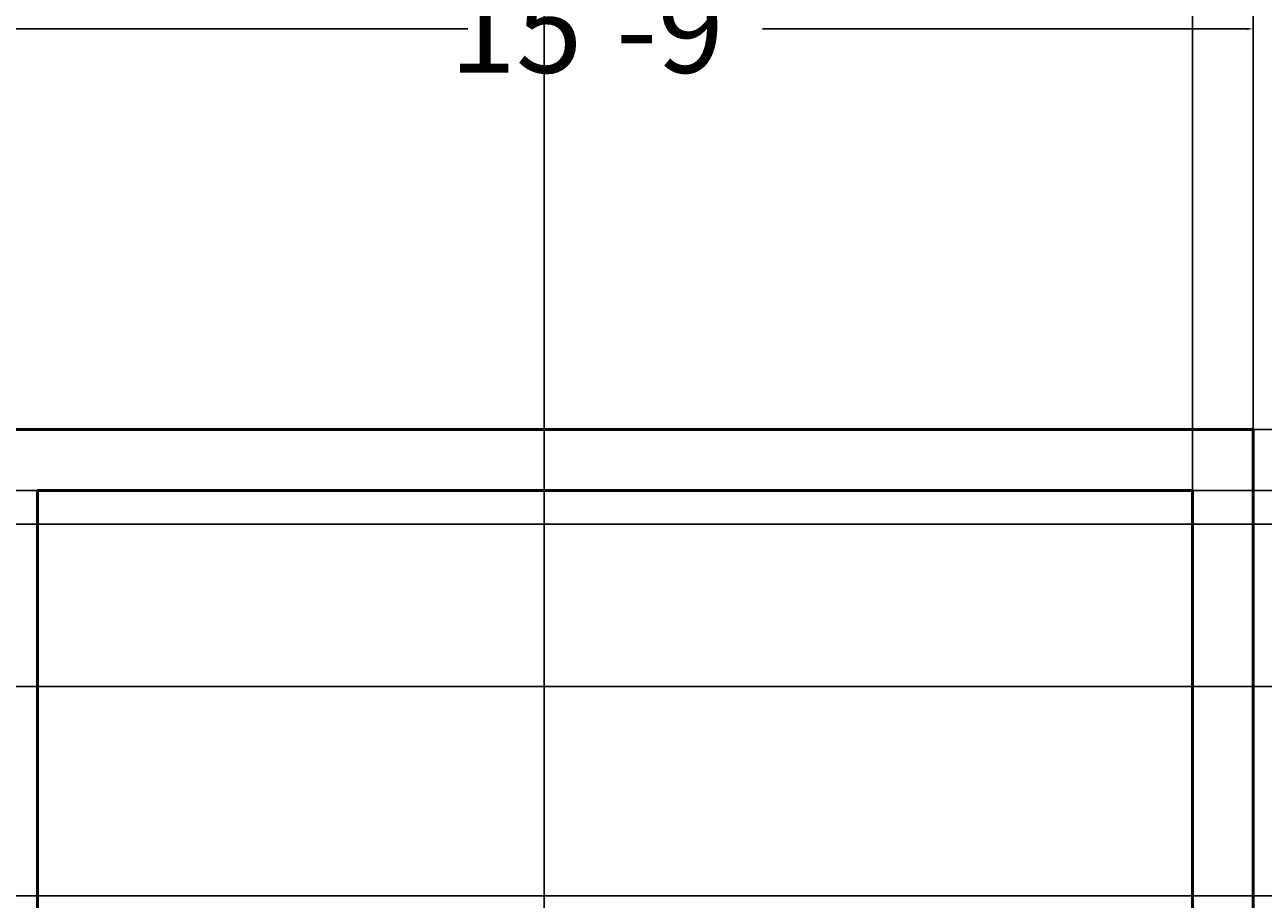
# Model space of a CAD drawing. Units: inches. Extents: x -364 to 705, y -52 to 1250.
# Tile 32 of 34: x 366 to 549, y 917 to 1046. Entities that reach past the tile are written whole.
import ezdxf

# ---------------------------------------------------------------- set-up
doc = ezdxf.new("R2010")
doc.units = ezdxf.units.IN
doc.header["$MEASUREMENT"] = 0
doc.layers.add('A-ANNO-DIMS', color=4, linetype='Continuous', lineweight=18)
doc.layers.add('A-WALL', color=41, linetype='Continuous', lineweight=50)
doc.styles.get("Standard").update_dxf_attribs({"font": 'arial.ttf'})
doc.dimstyles.get("Standard").update_dxf_attribs({"dimtxt": 1, "dimasz": 1, "dimexe": 0.18, "dimexo": 0.0625, "dimgap": 0.09, "dimtad": 0, "dimtih": 1, "dimtoh": 1, "dimdec": 0, "dimzin": 0, "dimdsep": 46, "dimlunit": 3, "dimtxsty": 'Standard', "dimcen": 0.09, "dimadec": 0, "dimazin": 0, "dimtfac": 1, "dimtdec": 0, "dimtofl": 0, "dimtmove": 0, "dimatfit": 3, "dimfxl": 1, "dimtolj": 1, "dimtzin": 0, "dimarcsym": 0})

# ---------------------------------------------------------------- blocks, each defined once
blk = doc.blocks.new('*D23')
at = {"layer": 'A-ANNO-DIMS', "color": 0, "lineweight": -2, "transparency": 16777216}
for p, q in [((28.58, 986.18), (28.58, 1127.53)), ((29.58, 1127.35), (265.4, 1127.35)), ((546.58, 1127.35), (310.76, 1127.35)), ((547.58, 986.18), (547.58, 1127.53))]:
    blk.add_line(p, q, dxfattribs=at)
at = {"layer": 'A-ANNO-DIMS', "color": 0, "transparency": 16777216}
for points in [[(29.58, 1127.52), (29.58, 1127.18), (28.58, 1127.35)], [(546.58, 1127.52), (546.58, 1127.18), (547.58, 1127.35)]]:
    blk.add_solid(points, dxfattribs=at)
at = {"layer": 'Defpoints', "color": 0, "transparency": 16777216}
for p in [(547.58, 1127.35), (28.58, 986.11), (547.58, 986.11)]:
    blk.add_point(p, dxfattribs=at)
at = {"layer": 'A-ANNO-DIMS', "color": 0, "transparency": 16777216, "insert": (288.08, 1127.35), "char_height": 1, "attachment_point": 5}
blk.add_mtext('\\A1;{\\H13x;43\'-3"}', dxfattribs=at)
blk = doc.blocks.new('*D27')
at = {"layer": 'A-ANNO-DIMS', "color": 0, "lineweight": -2, "transparency": 16777216}
for p, q in [((358.58, 986.18), (358.58, 1045.59)), ((359.58, 1045.41), (431.27, 1045.41)), ((546.58, 1045.41), (474.89, 1045.41)), ((547.58, 986.18), (547.58, 1045.59))]:
    blk.add_line(p, q, dxfattribs=at)
at = {"layer": 'A-ANNO-DIMS', "color": 0, "transparency": 16777216}
for points in [[(359.58, 1045.57), (359.58, 1045.24), (358.58, 1045.41)], [(546.58, 1045.57), (546.58, 1045.24), (547.58, 1045.41)]]:
    blk.add_solid(points, dxfattribs=at)
at = {"layer": 'Defpoints', "color": 0, "transparency": 16777216}
for p in [(547.58, 1045.41), (358.58, 986.11), (547.58, 986.11)]:
    blk.add_point(p, dxfattribs=at)
at = {"layer": 'A-ANNO-DIMS', "color": 0, "transparency": 16777216, "insert": (453.08, 1045.41), "char_height": 1, "attachment_point": 5}
blk.add_mtext('\\A1;{\\H13x;15\'-9"}', dxfattribs=at)
blk = doc.blocks.new('*D84')
at = {"layer": 'A-ANNO-DIMS', "color": 0, "lineweight": -2, "transparency": 16777216}
for p, q in [((547.64, 986.11), (703.01, 986.11)), ((702.83, 985.11), (702.83, 904.72)), ((702.83, 823.11), (702.83, 903.51)), ((538.64, 822.11), (703.01, 822.11))]:
    blk.add_line(p, q, dxfattribs=at)
at = {"layer": 'A-ANNO-DIMS', "color": 0, "transparency": 16777216}
for points in [[(702.66, 985.11), (703, 985.11), (702.83, 986.11)], [(702.66, 823.11), (703, 823.11), (702.83, 822.11)]]:
    blk.add_solid(points, dxfattribs=at)
at = {"layer": 'Defpoints', "color": 0, "transparency": 16777216}
for p in [(547.58, 986.11), (702.83, 986.11), (538.58, 822.11)]:
    blk.add_point(p, dxfattribs=at)
at = {"layer": 'A-ANNO-DIMS', "color": 0, "transparency": 16777216, "insert": (702.83, 904.11), "char_height": 1, "attachment_point": 5}
blk.add_mtext('\\A1;13\'-8"', dxfattribs=at)
blk = doc.blocks.new('*D95')
at = {"layer": 'A-ANNO-DIMS', "color": 0, "lineweight": -2, "transparency": 16777216}
for p, q in [((103.64, 972.11), (703.01, 972.11)), ((702.83, 971.11), (702.83, 960.72)), ((702.83, 949.11), (702.83, 959.51)), ((103.64, 948.11), (703.01, 948.11))]:
    blk.add_line(p, q, dxfattribs=at)
at = {"layer": 'A-ANNO-DIMS', "color": 0, "transparency": 16777216}
for points in [[(702.66, 971.11), (703, 971.11), (702.83, 972.11)], [(702.66, 949.11), (703, 949.11), (702.83, 948.11)]]:
    blk.add_solid(points, dxfattribs=at)
at = {"layer": 'Defpoints', "color": 0, "transparency": 16777216}
for p in [(103.58, 972.11), (702.83, 972.11), (103.58, 948.11)]:
    blk.add_point(p, dxfattribs=at)
at = {"layer": 'A-ANNO-DIMS', "color": 0, "transparency": 16777216, "insert": (702.83, 960.11), "char_height": 1, "attachment_point": 5}
blk.add_mtext('\\A1;2\'-0"', dxfattribs=at)
blk = doc.blocks.new('*D96')
at = {"layer": 'A-ANNO-DIMS', "color": 0, "lineweight": -2, "transparency": 16777216}
for p, q in [((358.64, 977.11), (703.01, 977.11)), ((702.83, 976.11), (702.83, 947.72)), ((702.83, 918.11), (702.83, 946.51)), ((358.64, 917.11), (703.01, 917.11))]:
    blk.add_line(p, q, dxfattribs=at)
at = {"layer": 'A-ANNO-DIMS', "color": 0, "transparency": 16777216}
for points in [[(702.66, 976.11), (703, 976.11), (702.83, 977.11)], [(702.66, 918.11), (703, 918.11), (702.83, 917.11)]]:
    blk.add_solid(points, dxfattribs=at)
at = {"layer": 'Defpoints', "color": 0, "transparency": 16777216}
for p in [(358.58, 977.11), (358.58, 917.11), (702.83, 917.11)]:
    blk.add_point(p, dxfattribs=at)
at = {"layer": 'A-ANNO-DIMS', "color": 0, "transparency": 16777216, "insert": (702.83, 947.11), "char_height": 1, "attachment_point": 5}
blk.add_mtext('\\A1;5\'-0"', dxfattribs=at)
blk = doc.blocks.new('*D99')
at = {"layer": 'A-ANNO-DIMS', "color": 0, "lineweight": -2, "transparency": 16777216}
for p, q in [((442.58, 822.18), (442.58, 1141.54)), ((443.58, 1141.36), (489.16, 1141.36)), ((537.58, 1141.36), (492, 1141.36)), ((538.58, 822.18), (538.58, 1141.54))]:
    blk.add_line(p, q, dxfattribs=at)
at = {"layer": 'A-ANNO-DIMS', "color": 0, "transparency": 16777216}
for points in [[(443.58, 1141.53), (443.58, 1141.2), (442.58, 1141.36)], [(537.58, 1141.53), (537.58, 1141.2), (538.58, 1141.36)]]:
    blk.add_solid(points, dxfattribs=at)
at = {"layer": 'Defpoints', "color": 0, "transparency": 16777216}
for p in [(538.58, 1141.36), (442.58, 822.11), (538.58, 822.11)]:
    blk.add_point(p, dxfattribs=at)
at = {"layer": 'A-ANNO-DIMS', "color": 0, "transparency": 16777216, "insert": (490.58, 1141.36), "char_height": 1, "attachment_point": 5}
blk.add_mtext('\\A1;8\'-0"', dxfattribs=at)

msp = doc.modelspace()

# ---------------------------------------------------------------- linework, layer by layer
at = {"layer": 'A-WALL'}
for p, q in [((547.58, 986.11), (28.58, 986.11)), ((547.58, 11.11), (547.58, 986.11)), ((538.58, 977.11), (367.58, 977.11)), ((367.58, 831.11), (367.58, 977.11)), ((538.58, 831.11), (538.58, 977.11))]:
    msp.add_line(p, q, dxfattribs=at)

# ---------------------------------------------------------------- dimensions: what is measured, and where the dimension line sits
at = {"layer": 'A-ANNO-DIMS'}
dim = msp.add_linear_dim(base=(538.58, 1141.36), p1=(442.58, 822.11), p2=(538.58, 822.11), dimstyle='Standard', override={"dimdec": 1, "dimlfac": 1, "dimrnd": 0, "dimzin": 1, "dimdsep": 46, "dimlunit": 4, "dimfrac": 2}, dxfattribs=at)
dim.commit()
dim.dimension.update_dxf_attribs({"geometry": '*D99', "text_midpoint": (490.58, 1141.36)})
for base, p1, picture, middle in [((547.58, 1127.35), (28.58, 986.11), '*D23', (288.08, 1127.35)), ((547.58, 1045.41), (358.58, 986.11), '*D27', (453.08, 1045.41))]:
    dim = msp.add_linear_dim(base=base, p1=p1, p2=(547.58, 986.11), text='{\\H13x;<>}', dimstyle='Standard', override={"dimclrd": 0, "dimclre": 0, "dimclrt": 0}, dxfattribs=at)
    dim.commit()
    dim.dimension.update_dxf_attribs({"geometry": picture, "text_midpoint": middle})
for base, p1, p2, picture, middle in [((702.83, 986.11), (538.58, 822.11), (547.58, 986.11), '*D84', (702.83, 904.11)), ((702.83, 917.11), (358.58, 977.11), (358.58, 917.11), '*D96', (702.83, 947.11)), ((702.83, 972.11), (103.58, 948.11), (103.58, 972.11), '*D95', (702.83, 960.11))]:
    dim = msp.add_linear_dim(base=base, p1=p1, p2=p2, angle=90, dimstyle='Standard', override={"dimdec": 1, "dimlfac": 1, "dimrnd": 0, "dimzin": 1, "dimdsep": 46, "dimlunit": 4, "dimfrac": 2}, dxfattribs=at)
    dim.commit()
    dim.dimension.update_dxf_attribs({"geometry": picture, "text_midpoint": middle})

doc.saveas('drawing.dxf')
